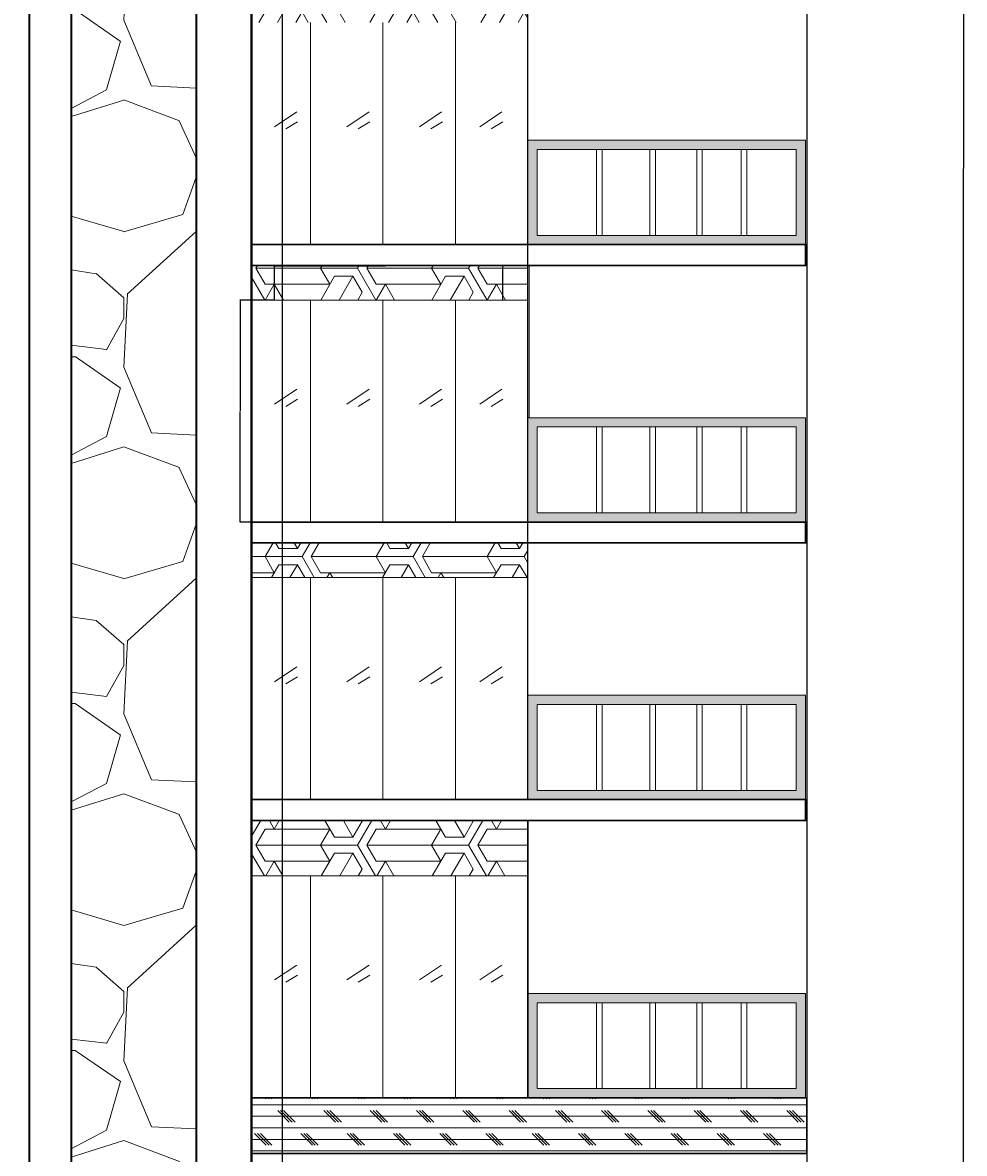
# Model space of a CAD drawing. Units: inches. Extents: x -38 to 698, y -57 to 1364.
# Tile 3 of 5: x 291 to 698, y 227 to 716. Entities that reach past the tile are written whole.
import ezdxf

# ---------------------------------------------------------------- set-up
doc = ezdxf.new("R2010")
doc.units = ezdxf.units.IN
doc.header["$MEASUREMENT"] = 0
for name, color, linetype, lineweight in [('A-ANNO-DIMS', 2, 'Continuous', 18), ('A-ELEV-PATT', 8, 'Continuous', 13), ('A-FLOR', 7, 'Continuous', 30), ('A-FLOR-HRAL', 7, 'Continuous', 20), ('A-GLAZ', 4, 'Continuous', 18), ('A-WALL', 7, 'Continuous', 35), ('A-WALL-PATT', 8, 'Continuous', 13)]:
    doc.layers.add(name, color=color, linetype=linetype, lineweight=lineweight)
doc.styles.get("Standard").update_dxf_attribs({"font": 'arial.ttf'})
doc.dimstyles.get("Standard").update_dxf_attribs({"dimtxt": 0.18, "dimasz": 0.18, "dimexe": 0.18, "dimexo": 0.0625, "dimgap": 0.09, "dimtad": 0, "dimtih": 1, "dimtoh": 1, "dimdec": 4, "dimzin": 0, "dimdsep": 46, "dimtxsty": 'Standard', "dimcen": 0.09, "dimadec": 0, "dimazin": 0, "dimtfac": 1, "dimtdec": 4, "dimtofl": 0, "dimtmove": 0, "dimatfit": 3, "dimfxl": 1, "dimtolj": 1, "dimtzin": 0, "dimarcsym": 0})

# ---------------------------------------------------------------- blocks, each defined once
blk = doc.blocks.new('WINDOW-4L-RH')
for p, q in [((15.6, 96), (15.6, 0)), ((46.9, 96), (46.9, 0)), ((78.2, 96), (78.2, 0)), ((0, 50.99), (9.6, 57.46)), ((31.3, 50.99), (40.9, 57.46)), ((62.61, 50.99), (72.2, 57.46)), ((88.7, 50.99), (98.29, 57.46)), ((4.92, 50.03), (9.96, 53.14)), ((36.22, 50.03), (41.26, 53.14)), ((67.52, 50.03), (72.56, 53.14)), ((93.62, 50.03), (98.65, 53.14))]:
    blk.add_line(p, q)
blk = doc.blocks.new('BALCONY-GUARD-PICKETS')
for p, q in [((0, 37.13), (0, 0)), ((2.41, 0), (2.41, 37.13)), ((19.25, 37.13), (19.25, 0)), ((21.65, 0), (21.65, 37.13)), ((39.53, 37.13), (39.53, 0)), ((41.93, 0), (41.93, 37.13)), ((62.55, 37.13), (62.55, 0)), ((64.96, 0), (64.96, 37.13))]:
    blk.add_line(p, q)
blk = doc.blocks.new('BALCONY-GUARD-PICKETS-BASE')
for p, q in [((19.25, 37.13), (19.25, 0)), ((21.65, 0), (21.65, 37.13)), ((39.53, 37.13), (39.53, 0)), ((41.93, 0), (41.93, 37.13)), ((62.55, 37.13), (62.55, 0)), ((64.96, 0), (64.96, 37.13))]:
    blk.add_line(p, q)
blk.add_lwpolyline([(0, 37.13), (0, 0), (2.41, 0), (2.41, 37.13)])
blk = doc.blocks.new('*D12')
at = {"layer": 'A-ANNO-DIMS', "color": 0, "lineweight": -2, "transparency": 16777216}
for p, q in [((399.56, 596.28), (399.56, 611.19)), ((399.74, 611.01), (447.56, 611.01)), ((498.03, 611.01), (450.21, 611.01)), ((498.21, 596.28), (498.21, 611.19))]:
    blk.add_line(p, q, dxfattribs=at)
at = {"layer": 'A-ANNO-DIMS', "color": 0, "transparency": 16777216}
for points in [[(399.74, 611.04), (399.74, 610.98), (399.56, 611.01)], [(498.03, 611.04), (498.03, 610.98), (498.21, 611.01)]]:
    blk.add_solid(points, dxfattribs=at)
at = {"layer": 'Defpoints', "color": 0, "transparency": 16777216}
for p in [(498.21, 611.01), (399.56, 596.21), (498.21, 596.21)]:
    blk.add_point(p, dxfattribs=at)
at = {"layer": 'A-ANNO-DIMS', "color": 0, "transparency": 16777216, "insert": (448.88, 611.01), "char_height": 0.18, "attachment_point": 5}
blk.add_mtext('\\A1;RH WINDOW 99 TYP.', dxfattribs=at)
blk = doc.blocks.new('*D13')
at = {"layer": 'A-ANNO-DIMS', "color": 0, "lineweight": -2, "transparency": 16777216}
for p, q in [((399.5, 596.21), (384.58, 596.21)), ((384.76, 596.03), (384.76, 548.4)), ((384.76, 500.39), (384.76, 548.03)), ((399.5, 500.21), (384.58, 500.21))]:
    blk.add_line(p, q, dxfattribs=at)
at = {"layer": 'A-ANNO-DIMS', "color": 0, "transparency": 16777216}
for points in [[(384.73, 596.03), (384.79, 596.03), (384.76, 596.21)], [(384.73, 500.39), (384.79, 500.39), (384.76, 500.21)]]:
    blk.add_solid(points, dxfattribs=at)
at = {"layer": 'Defpoints', "color": 0, "transparency": 16777216}
for p in [(384.76, 596.21), (399.56, 596.21), (399.56, 500.21)]:
    blk.add_point(p, dxfattribs=at)
at = {"layer": 'A-ANNO-DIMS', "color": 0, "transparency": 16777216, "insert": (384.76, 548.21), "char_height": 0.18, "attachment_point": 5}
blk.add_mtext('\\A1;96 TYP.', dxfattribs=at)
blk = doc.blocks.new('*D22')
at = {"layer": 'A-ANNO-DIMS', "color": 0, "lineweight": -2, "transparency": 16777216}
for p, q in [((29.69, 500.15), (29.69, -56.67)), ((629.69, 500.15), (629.69, -56.67)), ((29.87, -56.49), (329.4, -56.49)), ((629.51, -56.49), (329.97, -56.49))]:
    blk.add_line(p, q, dxfattribs=at)
at = {"layer": 'A-ANNO-DIMS', "color": 0, "transparency": 16777216}
for points in [[(29.87, -56.46), (29.87, -56.52), (29.69, -56.49)], [(629.51, -56.46), (629.51, -56.52), (629.69, -56.49)]]:
    blk.add_solid(points, dxfattribs=at)
at = {"layer": 'Defpoints', "color": 0, "transparency": 16777216}
for p in [(29.69, 500.21), (629.69, 500.21), (629.69, -56.49)]:
    blk.add_point(p, dxfattribs=at)
at = {"layer": 'A-ANNO-DIMS', "color": 0, "transparency": 16777216, "insert": (329.69, -56.49), "char_height": 0.18, "attachment_point": 5}
blk.add_mtext('\\A1;600', dxfattribs=at)
blk = doc.blocks.new('*D23')
at = {"layer": 'A-ANNO-DIMS', "color": 0, "lineweight": -2, "transparency": 16777216}
for p, q in [((595.72, 1295.04), (697.57, 1295.04)), ((697.39, 1294.86), (697.39, 653.31)), ((697.39, 11.39), (697.39, 652.94)), ((629.75, 11.21), (697.57, 11.21))]:
    blk.add_line(p, q, dxfattribs=at)
at = {"layer": 'A-ANNO-DIMS', "color": 0, "transparency": 16777216}
for points in [[(697.36, 1294.86), (697.42, 1294.86), (697.39, 1295.04)], [(697.36, 11.39), (697.42, 11.39), (697.39, 11.21)]]:
    blk.add_solid(points, dxfattribs=at)
at = {"layer": 'Defpoints', "color": 0, "transparency": 16777216}
for p in [(595.66, 1295.04), (697.39, 1295.04), (629.69, 11.21)]:
    blk.add_point(p, dxfattribs=at)
at = {"layer": 'A-ANNO-DIMS', "color": 0, "transparency": 16777216, "insert": (697.39, 653.13), "char_height": 0.18, "attachment_point": 5}
blk.add_mtext('\\A1;1283.8', dxfattribs=at)
blk = doc.blocks.new('*D25')
at = {"layer": 'A-ANNO-DIMS', "color": 0, "lineweight": -2, "transparency": 16777216}
for p, q in [((269.69, 1100.15), (269.69, -56.67)), ((389.69, 1100.15), (389.69, -56.67)), ((269.87, -56.49), (329.41, -56.49)), ((389.51, -56.49), (329.97, -56.49))]:
    blk.add_line(p, q, dxfattribs=at)
at = {"layer": 'A-ANNO-DIMS', "color": 0, "transparency": 16777216}
for points in [[(269.87, -56.46), (269.87, -56.52), (269.69, -56.49)], [(389.51, -56.46), (389.51, -56.52), (389.69, -56.49)]]:
    blk.add_solid(points, dxfattribs=at)
at = {"layer": 'Defpoints', "color": 0, "transparency": 16777216}
for p in [(269.69, 1100.21), (389.69, 1100.21), (389.69, -56.49)]:
    blk.add_point(p, dxfattribs=at)
at = {"layer": 'A-ANNO-DIMS', "color": 0, "transparency": 16777216, "insert": (329.69, -56.49), "char_height": 0.18, "attachment_point": 5}
blk.add_mtext('\\A1;120', dxfattribs=at)
blk = doc.blocks.new('*D26')
at = {"layer": 'A-ANNO-DIMS', "color": 0, "lineweight": -2, "transparency": 16777216}
for p, q in [((389.69, 1100.15), (389.69, -56.67)), ((629.69, 1100.15), (629.69, -56.67)), ((389.87, -56.49), (509.4, -56.49)), ((629.51, -56.49), (509.98, -56.49))]:
    blk.add_line(p, q, dxfattribs=at)
at = {"layer": 'A-ANNO-DIMS', "color": 0, "transparency": 16777216}
for points in [[(389.87, -56.46), (389.87, -56.52), (389.69, -56.49)], [(629.51, -56.46), (629.51, -56.52), (629.69, -56.49)]]:
    blk.add_solid(points, dxfattribs=at)
at = {"layer": 'Defpoints', "color": 0, "transparency": 16777216}
for p in [(389.69, 1100.21), (629.69, 1100.21), (629.69, -56.49)]:
    blk.add_point(p, dxfattribs=at)
at = {"layer": 'A-ANNO-DIMS', "color": 0, "transparency": 16777216, "insert": (509.69, -56.49), "char_height": 0.18, "attachment_point": 5}
blk.add_mtext('\\A1;240', dxfattribs=at)
blk = doc.blocks.new('*D28')
at = {"layer": 'A-ANNO-DIMS', "color": 0, "lineweight": -2, "transparency": 16777216}
for p, q in [((389.69, 380.28), (389.69, 1362.92)), ((389.87, 1362.74), (448.92, 1362.74)), ((508.88, 1362.74), (449.83, 1362.74)), ((509.06, 380.28), (509.06, 1362.92))]:
    blk.add_line(p, q, dxfattribs=at)
at = {"layer": 'A-ANNO-DIMS', "color": 0, "transparency": 16777216}
for points in [[(389.87, 1362.77), (389.87, 1362.71), (389.69, 1362.74)], [(508.88, 1362.77), (508.88, 1362.71), (509.06, 1362.74)]]:
    blk.add_solid(points, dxfattribs=at)
at = {"layer": 'Defpoints', "color": 0, "transparency": 16777216}
for p in [(509.06, 1362.74), (389.69, 380.21), (509.06, 380.21)]:
    blk.add_point(p, dxfattribs=at)
at = {"layer": 'A-ANNO-DIMS', "color": 0, "transparency": 16777216, "insert": (449.37, 1362.74), "char_height": 0.18, "attachment_point": 5}
blk.add_mtext('\\A1;119.38', dxfattribs=at)
blk = doc.blocks.new('*D48')
at = {"layer": 'A-ANNO-DIMS', "color": 0, "lineweight": -2, "transparency": 16777216}
for p, q in [((255.72, 101.28), (255.72, 1362.92)), ((255.9, 1362.74), (328.99, 1362.74)), ((402.85, 1362.74), (329.76, 1362.74)), ((403.03, 101.28), (403.03, 1362.92))]:
    blk.add_line(p, q, dxfattribs=at)
at = {"layer": 'A-ANNO-DIMS', "color": 0, "transparency": 16777216}
for points in [[(255.9, 1362.77), (255.9, 1362.71), (255.72, 1362.74)], [(402.85, 1362.77), (402.85, 1362.71), (403.03, 1362.74)]]:
    blk.add_solid(points, dxfattribs=at)
at = {"layer": 'Defpoints', "color": 0, "transparency": 16777216}
for p in [(403.03, 1362.74), (255.72, 101.21), (403.03, 101.21)]:
    blk.add_point(p, dxfattribs=at)
at = {"layer": 'A-ANNO-DIMS', "color": 0, "transparency": 16777216, "insert": (329.37, 1362.74), "char_height": 0.18, "attachment_point": 5}
blk.add_mtext('\\A1;147.3', dxfattribs=at)
blk = doc.blocks.new('*D51')
at = {"layer": 'A-ANNO-DIMS', "color": 0, "lineweight": -2, "transparency": 16777216}
for p, q in [((365.69, 1294.97), (365.69, -56.67)), ((389.69, 1258.97), (389.69, -56.67)), ((365.87, -56.49), (377.47, -56.49)), ((389.51, -56.49), (377.91, -56.49))]:
    blk.add_line(p, q, dxfattribs=at)
at = {"layer": 'A-ANNO-DIMS', "color": 0, "transparency": 16777216}
for points in [[(365.87, -56.46), (365.87, -56.52), (365.69, -56.49)], [(389.51, -56.46), (389.51, -56.52), (389.69, -56.49)]]:
    blk.add_solid(points, dxfattribs=at)
at = {"layer": 'Defpoints', "color": 0, "transparency": 16777216}
for p in [(365.69, 1295.04), (389.69, 1259.04), (389.69, -56.49)]:
    blk.add_point(p, dxfattribs=at)
at = {"layer": 'A-ANNO-DIMS', "color": 0, "transparency": 16777216, "insert": (377.69, -56.49), "char_height": 0.18, "attachment_point": 5}
blk.add_mtext('\\A1;24', dxfattribs=at)

msp = doc.modelspace()

# ---------------------------------------------------------------- hatches: boundary and pattern name
at = {"layer": 'A-ELEV-PATT', "transparency": 33554562}
h = msp.add_hatch(dxfattribs=at)
h.set_pattern_fill('HONEY', color=256, scale=40)
h.set_pattern_definition([(0, (-116.5534, -96.733), (7.5, 4.330127), [5, -10]), (120, (-116.5534, -96.733), (-7.5, 4.330127), [5, -10]), (60, (-116.5534, -96.733), (2e-15, 8.660254), [-10, 5])])
h.paths.add_polyline_path([(629.0638, 1145.3406), (509.0638, 1145.3406), (509.0638, 1100.2149), (629.0638, 1100.2149)])
h.paths.add_polyline_path([(625.0638, 1141.3406), (625.0638, 1104.2149), (513.0638, 1104.2149), (513.0638, 1141.3406)], flags=16)
h.paths.add_polyline_path([(629.0638, 1025.3406), (509.0638, 1025.3406), (509.0638, 980.2149), (629.0638, 980.2149)])
h.paths.add_polyline_path([(625.0638, 1021.3406), (625.0638, 984.2149), (513.0638, 984.2149), (513.0638, 1021.3406)], flags=16)
h.paths.add_polyline_path([(629.0638, 905.3406), (509.0638, 905.3406), (509.0638, 860.2149), (629.0638, 860.2149)])
h.paths.add_polyline_path([(625.0638, 901.3406), (625.0638, 864.2149), (513.0638, 864.2149), (513.0638, 901.3406)], flags=16)
h.paths.add_polyline_path([(629.0638, 785.3406), (509.0638, 785.3406), (509.0638, 740.2149), (629.0638, 740.2149)])
h.paths.add_polyline_path([(625.0638, 781.3406), (625.0638, 744.2149), (513.0638, 744.2149), (513.0638, 781.3406)], flags=16)
h.paths.add_polyline_path([(629.0638, 665.3406), (509.0638, 665.3406), (509.0638, 620.2149), (629.0638, 620.2149)])
h.paths.add_polyline_path([(625.0638, 661.3406), (625.0638, 624.2149), (513.0638, 624.2149), (513.0638, 661.3406)], flags=16)
h.paths.add_polyline_path([(629.0638, 545.3406), (509.0638, 545.3406), (509.0638, 500.2149), (629.0638, 500.2149)])
h.paths.add_polyline_path([(625.0638, 541.3406), (625.0638, 504.2149), (513.0638, 504.2149), (513.0638, 541.3406)], flags=16)
h.paths.add_polyline_path([(629.0638, 425.3406), (509.0638, 425.3406), (509.0638, 380.2149), (629.0638, 380.2149)])
h.paths.add_polyline_path([(625.0638, 421.3406), (625.0638, 384.2149), (513.0638, 384.2149), (513.0638, 421.3406)], flags=16)
h.paths.add_polyline_path([(629.0638, 296.3406), (509.0638, 296.3406), (509.0638, 251.2149), (629.0638, 251.2149)])
h.paths.add_polyline_path([(625.0638, 292.3406), (625.0638, 255.2149), (513.0638, 255.2149), (513.0638, 292.3406)], flags=16)
h.paths.add_polyline_path([(149.6854, 296.3406), (29.6854, 296.3406), (29.6854, 251.2149), (149.6854, 251.2149)])
h.paths.add_polyline_path([(145.6854, 292.3406), (145.6854, 255.2149), (33.6854, 255.2149), (33.6854, 292.3406)], flags=16)
h.paths.add_polyline_path([(149.6854, 425.3406), (29.6854, 425.3406), (29.6854, 380.2149), (149.6854, 380.2149)])
h.paths.add_polyline_path([(145.6854, 421.3406), (145.6854, 384.2149), (33.6854, 384.2149), (33.6854, 421.3406)], flags=16)
h.paths.add_polyline_path([(149.6854, 545.3406), (29.6854, 545.3406), (29.6854, 500.2149), (149.6854, 500.2149)])
h.paths.add_polyline_path([(33.6854, 504.2149), (33.6854, 541.3406), (145.6854, 541.3406), (145.6854, 504.2149)], flags=16)
h.paths.add_polyline_path([(149.6854, 665.3406), (29.6854, 665.3406), (29.6854, 620.2149), (149.6854, 620.2149)])
h.paths.add_polyline_path([(33.6854, 624.2149), (33.6854, 661.3406), (145.6854, 661.3406), (145.6854, 624.2149)], flags=16)
h.paths.add_polyline_path([(149.6854, 785.3406), (29.6854, 785.3406), (29.6854, 740.2149), (149.6854, 740.2149)])
h.paths.add_polyline_path([(33.6854, 744.2149), (33.6854, 781.3406), (145.6854, 781.3406), (145.6854, 744.2149)], flags=16)
h.paths.add_polyline_path([(149.6854, 905.3406), (29.6854, 905.3406), (29.6854, 860.2149), (149.6854, 860.2149)])
h.paths.add_polyline_path([(145.6854, 901.3406), (145.6854, 864.2149), (33.6854, 864.2149), (33.6854, 901.3406)], flags=16)
h.paths.add_polyline_path([(149.6854, 1025.3406), (29.6854, 1025.3406), (29.6854, 980.2149), (149.6854, 980.2149)])
h.paths.add_polyline_path([(33.6854, 984.2149), (33.6854, 1021.3406), (145.6854, 1021.3406), (145.6854, 984.2149)], flags=16)
h.paths.add_polyline_path([(149.6854, 1145.3406), (29.6854, 1145.3406), (29.6854, 1100.2149), (149.6854, 1100.2149)])
h.paths.add_polyline_path([(33.6854, 1104.2149), (33.6854, 1141.3406), (145.6854, 1141.3406), (145.6854, 1104.2149)], flags=16)
h = msp.add_hatch(dxfattribs=at)
h.set_pattern_fill('CORK', color=256, scale=40)
h.set_pattern_definition([(0, (-116.5534, -96.733), (0, 5), []), (135, (-114.053, -99.233), (-10, -10), [7.07107, -7.07107]), (135, (-112.803, -99.233), (-10, -10), [7.07107, -7.07107]), (135, (-111.553, -99.233), (-10, -10), [7.07107, -7.07107])])
h.paths.add_polyline_path([(269.6854, 131.2149), (29.6854, 131.2149), (29.6854, 107.2149), (269.6854, 107.2149)])
h.paths.add_polyline_path([(269.6854, 251.2149), (29.6854, 251.2149), (29.6854, 227.2149), (269.6854, 227.2149)])
h.paths.add_polyline_path([(629.6854, 251.2149), (389.6854, 251.2149), (389.6854, 227.2149), (629.6854, 227.2149)])
h.paths.add_polyline_path([(629.6854, 131.2149), (389.6854, 131.2149), (389.6854, 107.2149), (409.029, 107.2149), (629.6854, 107.2149)])
at = {"layer": 'A-WALL-PATT', "transparency": 33554625}
h = msp.add_hatch(dxfattribs=at)
h.set_pattern_fill('GRAVEL', color=256, scale=150)
h.set_pattern_definition([(228.0128, (-8.553, 53.267), (-1200, -1350), [20.1804, -1997.863]), (184.96974, (-22.0534, 38.267), (1800, 150), [34.63, -3428.3887]), (132.51045, (-56.553, 35.267), (1500, -1650), [24.418, -2417.405]), (267.2737, (-115.0534, -2.233), (150, 3000), [31.5357, -3122.0337]), (292.83365, (-116.5534, -33.733), (-750, 1800), [30.923, -3061.406]), (357.2737, (-104.5534, -62.233), (-3000, 150), [31.5357, -3122.0337]), (37.69424, (-73.0534, -63.733), (-1950, -1500), [41.7043, -4128.7273]), (72.25533, (-40.0534, -38.233), (1050, 3300), [39.373, -3897.9482]), (121.42957, (-28.0534, -0.733), (-1200, 1950), [31.6425, -3132.611]), (175.2364, (-44.553, 26.267), (1650, -150), [36.125, -1770.1144]), (222.39744, (-80.5534, 29.267), (-1800, -1650), [46.7172, -4625.0063]), (138.8141, (33.447, -3.733), (-1050, 900), [15.945, -1578.577]), (171.4692, (21.447, 6.767), (1950, -300), [30.3356, -3003.2267]), (225, (-8.55, 11.27), (-2e-14, -150), [21.213, -190.919]), (203.1986, (-19.053, 29.267), (750, 300), [11.424, -1130.942]), (291.8014, (-29.553, 24.767), (-150, 450), [16.155, -791.619]), (30.9638, (-23.553, 9.767), (450, 300), [26.239, -848.403]), (161.565, (-1.053, 23.267), (300, -150), [18.974, -455.368]), (16.38954, (-116.553, 24.767), (1500, 450), [26.58, -2631.427]), (70.3462, (-91.053, 32.267), (-600, -1650), [22.299, -2207.611]), (293.1986, (-1.053, 53.267), (-300, 750), [22.847, -1119.519]), (343.6105, (7.947, 32.267), (-1500, 450), [26.58, -2631.427]), (339.444, (-116.553, -68.233), (-750, 300), [25.632, -1255.9686]), (294.7751, (-92.553, -77.233), (-750, 1650), [21.477, -2126.1965]), (66.8014, (0.447, -96.733), (300, 750), [22.847, -1119.519]), (17.354, (9.447, -75.733), (-1950, -600), [25.1446, -2489.3135]), (69.444, (-73.053, -96.733), (-300, -750), [12.816, -1268.7846]), (101.31, (-8.553, -96.733), (-150, 600), [7.649, -757.204]), (165.9638, (-10.053, -89.233), (450, -150), [30.923, -587.543]), (186.009, (-40.053, -81.733), (1500, 150), [28.6575, -2837.0885]), (303.69, (-23.553, -3.733), (-150, 300), [21.633, -519.2]), (353.1572, (-11.5534, -21.733), (2550, -300), [37.769, -3739.1344]), (60.9454, (25.947, -26.233), (-600, -1050), [15.443, -1528.901]), (90, (33.45, -12.73), (-150, 150), [9, -141]), (120.2564, (-43.053, -77.233), (600, -1050), [20.8386, -2063.028]), (48.0128, (-53.553, -59.233), (1200, 1350), [40.361, -1977.683]), (0, (-26.55, -29.23), (150, 150), [39, -111]), (325.30485, (12.447, -29.233), (1500, -1050), [23.717, -2347.991]), (254.0546, (31.947, -42.733), (-150, -600), [21.84, -1070.176]), (207.646, (25.9466, -63.733), (-2850, -1500), [35.5598, -3520.421]), (175.4261, (-5.5534, -80.233), (-1950, 150), [37.62, -3724.361])])
h.paths.add_polyline_path([(311.6854, 107.2149), (365.6854, 107.2149), (365.6854, 851.2149), (365.6854, 971.2149), (365.6854, 1091.2149), (365.6854, 1140.6923), (311.6854, 1140.6923), (311.6854, 971.2149), (311.6854, 851.2149)])
at = {"layer": 'A-WALL-PATT', "transparency": 33554562}
h = msp.add_hatch(dxfattribs=at)
h.set_pattern_fill('ESCHER', color=256, scale=40)
h.set_pattern_definition([(60, (-116.553, -96.733), (-48, -1e-08), [44, -4]), (180, (-116.553, -96.733), (24, -41.5692), [44, -4]), (300, (-116.553, -96.733), (48, -1e-08), [44, -4]), (60, (-112.553, -96.733), (-48, -1e-08), [8, -40]), (300, (-112.553, -96.733), (48, -1e-08), [8, -40]), (60, (-118.553, -93.27), (-48, -1e-08), [8, -40]), (180, (-118.553, -93.27), (24, -41.5692), [8, -40]), (300, (-118.553, -100.197), (48, -1e-08), [8, -40]), (180, (-118.553, -100.197), (24, -41.5692), [8, -40]), (60, (-132.553, -96.733), (-48, -1e-08), [8, -40]), (300, (-132.553, -96.733), (48, -1e-08), [8, -40]), (60, (-108.553, -110.59), (-48, -1e-08), [8, -40]), (180, (-108.553, -110.59), (24, -41.5692), [8, -40]), (300, (-108.553, -82.877), (48, -1e-08), [8, -40]), (180, (-108.553, -82.877), (24, -41.5692), [8, -40]), (0, (-108.553, -89.805), (-24, 41.5692), [28, -20]), (0, (-108.553, -103.66), (-24, 41.5692), [28, -20]), (120, (-114.553, -86.34), (-48, 1e-08), [28, -20]), (120, (-126.553, -93.27), (-48, 1e-08), [28, -20]), (240, (-126.553, -100.197), (24, -41.5692), [28, -20]), (240, (-114.553, -107.125), (24, -41.5692), [28, -20])])
h.paths.add_polyline_path([(269.6854, 371.2149), (149.6854, 371.2149), (149.6854, 347.2149), (269.6854, 347.2149)])
h.paths.add_polyline_path([(509.0638, 371.2149), (389.6854, 371.2149), (389.6854, 347.2149), (509.0638, 347.2149)])
h.paths.add_polyline_path([(269.6854, 491.2149), (149.6854, 491.2149), (149.6854, 476.2149), (269.6854, 476.2149)])
h.paths.add_polyline_path([(509.0638, 491.2149), (389.6854, 491.2149), (389.6854, 476.2149), (509.0638, 476.2149)])
h.paths.add_polyline_path([(509.0638, 611.2149), (389.6854, 611.2149), (389.6854, 596.2149), (509.0638, 596.2149)])
h.paths.add_polyline_path([(269.6854, 611.2149), (149.6854, 611.2149), (149.6854, 596.2149), (269.6854, 596.2149)])
h.paths.add_polyline_path([(269.6854, 731.2149), (149.6854, 731.2149), (149.6854, 716.2149), (269.6854, 716.2149)])
h.paths.add_polyline_path([(509.0638, 731.2149), (389.6854, 731.2149), (389.6854, 716.2149), (509.0638, 716.2149)])
h.paths.add_polyline_path([(509.0638, 851.2149), (389.6854, 851.2149), (389.6854, 836.2149), (509.0638, 836.2149)])
h.paths.add_polyline_path([(269.6854, 851.2149), (149.6854, 851.2149), (149.6854, 836.2149), (269.6854, 836.2149)])
h.paths.add_polyline_path([(269.6854, 971.2149), (149.6854, 971.2149), (149.6854, 956.2149), (269.6854, 956.2149)])
h.paths.add_polyline_path([(509.0638, 971.2149), (389.6854, 971.2149), (389.6854, 956.2149), (509.0638, 956.2149)])
h.paths.add_polyline_path([(509.0638, 1091.2149), (389.6854, 1091.2149), (389.6854, 1076.2149), (509.0638, 1076.2149)])
h.paths.add_polyline_path([(269.6854, 1091.2149), (149.6854, 1091.2149), (149.6854, 1076.2149), (269.6854, 1076.2149)])

# ---------------------------------------------------------------- linework, layer by layer
at = {"layer": 'A-FLOR'}
for points in [[(629.6854, 611.2149), (389.6854, 611.2149), (629.6854, 611.2149), (629.6854, 620.2149), (389.6854, 620.2149)], [(629.0638, 620.2149), (389.6854, 620.2149), (629.0638, 620.2149), (629.0638, 611.2149), (389.6854, 611.2149), (629.0638, 611.2149)], [(629.6854, 491.2149), (389.6854, 491.2149), (629.6854, 491.2149), (629.6854, 500.2149), (389.6854, 500.2149)], [(629.0638, 500.2149), (389.6854, 500.2149), (629.0638, 500.2149), (629.0638, 491.2149), (389.6854, 491.2149), (629.0638, 491.2149)], [(629.6854, 371.2149), (389.6854, 371.2149), (629.6854, 371.2149), (629.6854, 380.2149), (389.6854, 380.2149)], [(629.0638, 380.2149), (389.6854, 380.2149), (629.0638, 380.2149), (629.0638, 371.2149), (509.0638, 371.2149)], [(629.0638, 371.2149), (389.6854, 371.2149), (509.0638, 371.2149), (509.0638, 251.2149)], [(629.0638, 227.2149), (389.6854, 227.2149), (629.6854, 227.2149), (629.6854, 251.2149), (389.6854, 251.2149), (629.6854, 251.2149)]]:
    msp.add_lwpolyline(points, dxfattribs=at)
msp.add_lwpolyline([(629.0638, 251.2149), (389.6854, 251.2149)], close=True, dxfattribs=at)
at = {"layer": 'A-FLOR-HRAL'}
for points in [[(509.0638, 665.3406), (629.0638, 665.3406), (629.0638, 620.2149), (509.0638, 620.2149)], [(513.0638, 661.3406), (625.0638, 661.3406), (625.0638, 624.2149), (513.0638, 624.2149)], [(509.0638, 545.3406), (629.0638, 545.3406), (629.0638, 500.2149), (509.0638, 500.2149)], [(513.0638, 541.3406), (625.0638, 541.3406), (625.0638, 504.2149), (513.0638, 504.2149)], [(509.0638, 425.3406), (629.0638, 425.3406), (629.0638, 380.2149), (509.0638, 380.2149)], [(513.0638, 421.3406), (625.0638, 421.3406), (625.0638, 384.2149), (513.0638, 384.2149)], [(509.0638, 296.3406), (629.0638, 296.3406), (629.0638, 251.2149), (509.0638, 251.2149)], [(513.0638, 292.3406), (625.0638, 292.3406), (625.0638, 255.2149), (513.0638, 255.2149)]]:
    msp.add_lwpolyline(points, close=True, dxfattribs=at)
at = {"layer": 'A-GLAZ'}
for p, q in [((509.0638, 596.2149), (389.6854, 596.2149)), ((509.0638, 476.2149), (389.6854, 476.2149)), ((509.0638, 347.2149), (389.6854, 347.2149))]:
    msp.add_line(p, q, dxfattribs=at)
for points in [[(509.0638, 620.2149), (509.0638, 731.2149), (509.0638, 620.2149), (509.0638, 500.2149), (509.0638, 611.2149)], [(509.6854, 545.3406), (509.6854, 611.2149)]]:
    msp.add_lwpolyline(points, dxfattribs=at)
msp.add_lwpolyline([(509.0638, 380.2149), (509.0638, 491.2149)], close=True, dxfattribs=at)
at = {"layer": 'A-WALL'}
for points in [[(29.6854, 131.2149), (269.6854, 131.2149), (29.6854, 131.2149), (29.6854, 107.2149), (389.6854, 107.2149), (389.6854, 851.2149), (389.6854, 971.2149), (389.6854, 1091.2149), (389.6854, 1259.0353), (595.6569, 1259.0353), (595.6569, 1295.0353), (365.6854, 1295.0353), (365.6854, 1211.2149), (365.6854, 1091.2149), (365.6854, 971.2149), (365.6854, 851.2149), (365.6854, 107.2149)], [(293.6854, 107.2149), (293.6854, 851.2149), (293.6854, 971.2149), (293.6854, 1295.0353), (311.6854, 1295.0353), (311.6854, 1211.2149), (311.6854, 971.2149), (311.6854, 851.2149), (311.6854, 107.2149)]]:
    msp.add_lwpolyline(points, dxfattribs=at)

# ---------------------------------------------------------------- block references
at = {"layer": 'A-FLOR-HRAL', "rotation": 180}
for name, p in [('BALCONY-GUARD-PICKETS', (603.7292, 661.3405)), ('BALCONY-GUARD-PICKETS', (603.7292, 541.3405)), ('BALCONY-GUARD-PICKETS', (603.7292, 421.3405)), ('BALCONY-GUARD-PICKETS-BASE', (603.7292, 292.3405))]:
    msp.add_blockref(name, p, dxfattribs=at)
at = {"layer": 'A-GLAZ'}
for p in [(399.558, 620.215), (399.558, 500.215), (399.558, 380.215), (399.558, 251.215)]:
    msp.add_blockref('WINDOW-4L-RH', p, dxfattribs=at)

# ---------------------------------------------------------------- dimensions: what is measured, and where the dimension line sits
at = {"layer": 'A-ANNO-DIMS'}
for base, p1, p2, override, picture, middle in [((403.029, 1362.7353), (255.7202, 101.2149), (403.029, 101.2149), {"dimdec": 1, "dimlfac": 1, "dimrnd": 0, "dimzin": 0, "dimdsep": 46, "dimlunit": 2}, '*D48', (329.3746, 1362.7353)), ((509.0638, 1362.7353), (389.6854, 380.2149), (509.0638, 380.2149), {"dimdec": 2, "dimlfac": 1, "dimrnd": 0, "dimzin": 0, "dimdsep": 46, "dimlunit": 2}, '*D28', (449.3746, 1362.7353)), ((389.6854, -56.4851), (365.6854, 1295.0353), (389.6854, 1259.0353), {"dimdec": 0, "dimlfac": 1, "dimrnd": 0, "dimzin": 0, "dimdsep": 46, "dimlunit": 2}, '*D51', (377.6854, -56.4851)), ((389.6854, -56.4851), (269.6854, 1100.2149), (389.6854, 1100.2149), {"dimdec": 0, "dimlfac": 1, "dimrnd": 0, "dimzin": 0, "dimdsep": 46, "dimlunit": 2}, '*D25', (329.6854, -56.4851)), ((629.6854, -56.4851), (389.6854, 1100.2149), (629.6854, 1100.2149), {"dimdec": 0, "dimlfac": 1, "dimrnd": 0, "dimzin": 0, "dimdsep": 46, "dimlunit": 2}, '*D26', (509.6854, -56.4851)), ((629.6854, -56.4851), (29.6854, 500.2149), (629.6854, 500.2149), {"dimdec": 0, "dimlfac": 1, "dimrnd": 0, "dimzin": 0, "dimdsep": 46, "dimlunit": 2}, '*D22', (329.6854, -56.4851))]:
    dim = msp.add_linear_dim(base=base, p1=p1, p2=p2, dimstyle='Standard', override=override, dxfattribs=at)
    dim.commit()
    dim.dimension.update_dxf_attribs({"geometry": picture, "text_midpoint": middle})
dim = msp.add_linear_dim(base=(697.3854, 1295.0353), p1=(629.6854, 11.2149), p2=(595.6569, 1295.0353), angle=90, dimstyle='Standard', override={"dimdec": 1, "dimlfac": 1, "dimrnd": 0, "dimzin": 0, "dimdsep": 46, "dimlunit": 2}, dxfattribs=at)
dim.commit()
dim.dimension.update_dxf_attribs({"geometry": '*D23', "text_midpoint": (697.3854, 653.1251)})
dim = msp.add_linear_dim(base=(498.2117, 611.013), p1=(399.5579, 596.2149), p2=(498.2117, 596.2149), text='RH WINDOW <> TYP.', dimstyle='Standard', override={"dimdec": 0, "dimlfac": 1, "dimrnd": 0, "dimzin": 0, "dimdsep": 46, "dimlunit": 2}, dxfattribs=at)
dim.commit()
dim.dimension.update_dxf_attribs({"geometry": '*D12', "text_midpoint": (448.8848, 611.013)})
dim = msp.add_linear_dim(base=(384.7599, 596.2149), p1=(399.5579, 500.2149), p2=(399.5579, 596.2149), angle=90, text='<> TYP.', dimstyle='Standard', override={"dimdec": 0, "dimlfac": 1, "dimrnd": 0, "dimzin": 0, "dimdsep": 46, "dimlunit": 2}, dxfattribs=at)
dim.commit()
dim.dimension.update_dxf_attribs({"geometry": '*D13', "text_midpoint": (384.7599, 548.2149)})

doc.saveas('drawing.dxf')
